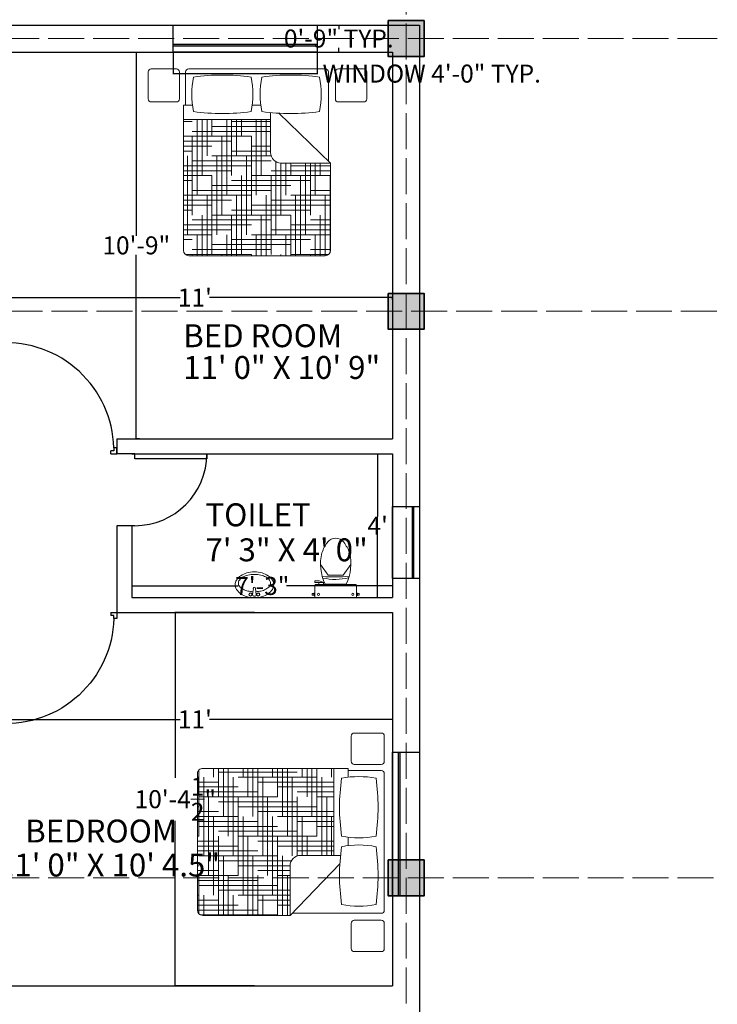
# Model space of a CAD drawing. Units: inches. Extents: x -113 to 5399, y -1393 to 3302.
# Tile 9 of 40: x 1194 to 1427, y 460 to 788. Entities that reach past the tile are written whole.
import ezdxf

# ---------------------------------------------------------------- set-up
doc = ezdxf.new("R2010")
doc.units = ezdxf.units.IN
doc.header["$MEASUREMENT"] = 0
doc.linetypes.add('ACAD_ISO02W100', pattern=[15, 12, -3])
for name, color, linetype, lineweight in [('A-ANNO-DIMS', 254, 'Continuous', 18), ('A-AREA-IDEN', 4, 'Continuous', 18), ('A-COLS', 7, 'Continuous', 35), ('A-FLOR-FIXT', 8, 'Continuous', 18), ('doors', 2, 'Continuous', 25), ('furniture', 131, 'Continuous', 18), ('GRIDS', 7, 'ACAD_ISO02W100', 13), ('walls', 1, 'Continuous', 25), ('windows', 3, 'Continuous', 25)]:
    doc.layers.add(name, color=color, linetype=linetype, lineweight=lineweight)
doc.styles.get("Standard").update_dxf_attribs({"font": 'arial.ttf'})
doc.dimstyles.get("Standard").update_dxf_attribs({"dimtxt": 6, "dimasz": 0.18, "dimexe": 0.18, "dimexo": 0.0625, "dimgap": 0.09, "dimtad": 0, "dimtih": 1, "dimtoh": 1, "dimdec": 1, "dimzin": 0, "dimdsep": 46, "dimlunit": 4, "dimtxsty": 'Standard', "dimblk": 'ARCHTICK', "dimcen": 0.09, "dimadec": 0, "dimazin": 0, "dimtfac": 1, "dimtdec": 1, "dimtofl": 0, "dimtmove": 0, "dimatfit": 3, "dimfxl": 1, "dimtolj": 1, "dimtzin": 0, "dimarcsym": 0})

# ---------------------------------------------------------------- blocks, each defined once
blk = doc.blocks.new('*U2')
for p, q in [((0, 0), (0, -6)), ((24, 0), (24, -6))]:
    blk.add_line(p, q)
blk.add_lwpolyline([(0, 0), (0, 24), (1.75, 24), (1.75, 0)], close=True)
blk.add_arc((0, 0), 24, 0, 90)
blk = doc.blocks.new('*X4')
at = {"color": 0}
for p, q in [((4.3594, 18.5625), (4.3594, 18.6457)), ((4.5, 18), (4.5, 18.6457)), ((4.5469, 18.1875), (4.5469, 18.6457)), ((4.5938, 18.375), (4.5938, 18.6457)), ((4.6406, 18.5625), (4.6406, 18.6457)), ((4.6875, 18.6094), (5.4375, 18.6094)), ((4.7812, 18), (4.7812, 18.6457)), ((4.8281, 18.1875), (4.8281, 18.6457)), ((4.875, 18.375), (4.875, 18.6457)), ((4.9219, 18.5625), (4.9219, 18.6457)), ((5.0625, 18), (5.0625, 18.6457)), ((5.1094, 18.1875), (5.1094, 18.6457)), ((5.1562, 18.375), (5.1562, 18.6457)), ((5.2031, 18.5625), (5.2031, 18.6457)), ((5.3438, 18), (5.3438, 18.6457)), ((5.3906, 18.1875), (5.3906, 18.6457)), ((5.4375, 18.375), (5.4375, 18.6457)), ((5.4844, 18.5625), (5.4844, 18.6457)), ((5.625, 18), (5.625, 18.6287)), ((4.3395, 18.5156), (5.0625, 18.5156)), ((4.4531, 17.8169), (4.4531, 18.5625)), ((4.5, 18.5625), (5.25, 18.5625)), ((4.7344, 17.8125), (4.7344, 18.5625)), ((5.0156, 17.8125), (5.0156, 18.5625)), ((5.2969, 17.8125), (5.2969, 18.5625)), ((5.4375, 18.5156), (5.6375, 18.5156)), ((5.5781, 17.8125), (5.5781, 18.5625)), ((5.625, 18.5625), (5.6375, 18.5625)), ((4.3395, 18.4688), (4.875, 18.4688)), ((4.3395, 18.4219), (4.6875, 18.4219)), ((5.0625, 18.4219), (5.6375, 18.4219)), ((5.25, 18.4688), (5.6375, 18.4688)), ((4.3395, 18.375), (4.5, 18.375)), ((4.4062, 17.8169), (4.4062, 18.375)), ((4.6875, 17.8114), (4.6875, 18.375)), ((4.6875, 18.3281), (5.4375, 18.3281)), ((4.875, 18.375), (5.625, 18.375)), ((4.9688, 17.625), (4.9688, 18.375)), ((5.25, 17.625), (5.25, 18.375)), ((5.5312, 17.625), (5.5312, 18.375)), ((4.3395, 18.2344), (5.0625, 18.2344)), ((4.5, 18.2812), (5.25, 18.2812)), ((5.4375, 18.2344), (5.6375, 18.2344)), ((5.625, 18.2812), (5.6375, 18.2812)), ((4.3395, 18.1875), (4.875, 18.1875)), ((4.3395, 18.1406), (4.6875, 18.1406)), ((4.3594, 17.8169), (4.3594, 18.1875)), ((4.6406, 17.8169), (4.6406, 18.1875)), ((4.9219, 17.4375), (4.9219, 18.1875)), ((5.0625, 18.1406), (5.6375, 18.1406)), ((5.2031, 17.4375), (5.2031, 18.1875)), ((5.25, 18.1875), (5.6375, 18.1875)), ((5.4844, 17.4375), (5.4844, 18.1875)), ((4.3395, 18.0938), (4.5, 18.0938)), ((4.6875, 18.0469), (5.4375, 18.0469)), ((4.875, 18.0938), (5.625, 18.0938)), ((4.3395, 17.9531), (5.0625, 17.9531)), ((4.5, 18), (5.25, 18)), ((4.5938, 17.8169), (4.5938, 18)), ((4.875, 17.25), (4.875, 18)), ((5.1562, 17.25), (5.1562, 18)), ((5.4375, 17.25), (5.4375, 18)), ((5.4375, 17.9531), (5.6375, 17.9531)), ((5.625, 18), (5.6375, 18)), ((4.3395, 17.9062), (4.875, 17.9062)), ((4.3395, 17.8594), (4.6875, 17.8594)), ((5.0625, 17.8594), (5.6375, 17.8594)), ((5.25, 17.9062), (5.6375, 17.9062)), ((4.7421, 17.7656), (5.4375, 17.7656)), ((4.8281, 17.2457), (4.8281, 17.8125)), ((4.875, 17.8125), (5.625, 17.8125)), ((5.1094, 17.2457), (5.1094, 17.8125)), ((5.3906, 17.2457), (5.3906, 17.8125)), ((4.7548, 17.7188), (5.25, 17.7188)), ((4.7548, 17.6719), (5.0625, 17.6719)), ((5.4375, 17.6719), (5.6375, 17.6719)), ((5.625, 17.7188), (5.6375, 17.7188)), ((4.7548, 17.625), (4.875, 17.625)), ((4.7812, 17.2457), (4.7812, 17.625)), ((5.0625, 17.2457), (5.0625, 17.625)), ((5.0625, 17.5781), (5.6375, 17.5781)), ((5.25, 17.625), (5.6375, 17.625)), ((5.3438, 17.2457), (5.3438, 17.625)), ((5.625, 17.2627), (5.625, 17.625)), ((4.7548, 17.4844), (5.4375, 17.4844)), ((4.875, 17.5312), (5.625, 17.5312)), ((4.7548, 17.4375), (5.25, 17.4375)), ((4.7548, 17.3906), (5.0625, 17.3906)), ((5.0156, 17.2457), (5.0156, 17.4375)), ((5.2969, 17.2457), (5.2969, 17.4375)), ((5.4375, 17.3906), (5.6375, 17.3906)), ((5.5781, 17.2457), (5.5781, 17.4375)), ((5.625, 17.4375), (5.6375, 17.4375)), ((4.7548, 17.3438), (4.875, 17.3438)), ((5.0625, 17.2969), (5.6375, 17.2969)), ((5.25, 17.3438), (5.6375, 17.3438)), ((4.875, 17.25), (5.6077, 17.25)), ((4.9688, 17.2457), (4.9688, 17.25)), ((5.25, 17.2457), (5.25, 17.25)), ((5.5312, 17.2457), (5.5312, 17.25))]:
    blk.add_line(p, q, dxfattribs=at)
blk = doc.blocks.new('MAT-P01')
for p, q in [((0.0087, 0.8464), (0.2471, 0.8464)), ((0.3737, 0.8464), (1.6737, 0.8464)), ((1.7922, 0.8464), (2.0306, 0.8464)), ((-0.0213, 0.8164), (-0.0213, 0.5605)), ((0.2771, 0.8164), (0.2771, 0.5605)), ((0.3437, 0.8164), (0.3437, -0.0316)), ((1.7037, 0.8164), (1.7037, 0.5005)), ((1.7622, 0.8164), (1.7622, 0.5605)), ((2.0606, 0.8164), (2.0606, 0.5605)), ((0.0087, 0.5305), (0.2471, 0.5305)), ((0.9879, 0.5005), (1.0693, 0.5005)), ((1.6393, 0.5005), (1.7237, 0.5005)), ((1.7237, 0.5005), (1.7237, -0.8836)), ((1.7922, 0.5305), (2.0306, 0.5305)), ((0.8146, 0.423), (0.3237, -0.0509)), ((0.8949, 0.4293), (0.8949, 0.0491)), ((0.8949, 0.3643), (1.7237, 0.3643)), ((0.8949, 0.3643), (0.8949, 0.0491)), ((0.8949, 0.3643), (1.7237, 0.3643)), ((1.7237, 0.3643), (1.7237, -0.8836)), ((0.3237, -0.0509), (0.7949, -0.0509)), ((0.3237, -0.0509), (0.3237, -0.8836)), ((0.3737, -0.9336), (1.6737, -0.9336))]:
    blk.add_line(p, q)
for centre, radius, start, end in [((0.0087, 0.8164), 0.03, 90, 180), ((0.2471, 0.8164), 0.03, 0, 90), ((0.3737, 0.8164), 0.03, 90, 180), ((1.6737, 0.8164), 0.03, 0, 90), ((1.7922, 0.8164), 0.03, 90, 180), ((2.0306, 0.8164), 0.03, 0, 90), ((1.2251, 0.6034), 0.8138, 168.37298, 191.62702), ((0.7029, -1.1436), 1.9306, 81.81622, 98.18378), ((0.1806, 0.6034), 0.8138, 348.37298, 11.62702), ((1.8766, 0.6034), 0.8138, 168.37298, 191.62702), ((1.3543, -1.1436), 1.9306, 81.81622, 98.18378), ((0.8321, 0.6034), 0.8138, 348.37298, 11.62702), ((0.0087, 0.5605), 0.03, 180, 270), ((0.2471, 0.5605), 0.03, 270, 0), ((1.7922, 0.5605), 0.03, 180, 270), ((2.0306, 0.5605), 0.03, 270, 0), ((0.7029, 2.3504), 1.9306, 261.81622, 278.18378), ((1.3543, 2.3504), 1.9306, 261.81622, 278.18378), ((0.7949, 0.0491), 0.1, 270, 0), ((0.3737, -0.8836), 0.05, 180, 270), ((1.6737, -0.8836), 0.05, 270, 0)]:
    blk.add_arc(centre, radius, start, end)
at = {"rotation": 270}
blk.add_blockref('*X4', (-16.9221, 4.7038), dxfattribs=at)
blk = doc.blocks.new('toilet-3')
at = {"color": 0, "linetype": 'ByBlock'}
for p, q in [((-0.281, -0.05), (-0.281, -0.069)), ((-0.281, -0.05), (-0.261, -0.05)), ((-0.281, -0.069), (-0.261, -0.069)), ((-0.261, -0.047), (-0.261, -0.072)), ((-0.261, -0.047), (-0.251, -0.047)), ((-0.261, -0.072), (-0.251, -0.072)), ((-0.251, -0.047), (-0.251, -0.072)), ((-0.25, -0.03), (-0.25, -0.165)), ((0.24, -0.02), (-0.24, -0.02)), ((0.25, -0.03), (0.25, -0.165)), ((0.261, -0.047), (0.251, -0.047)), ((0.251, -0.047), (0.251, -0.072)), ((0.261, -0.072), (0.251, -0.072)), ((0.261, -0.047), (0.261, -0.072)), ((0.281, -0.05), (0.261, -0.05)), ((0.281, -0.069), (0.261, -0.069)), ((0.281, -0.05), (0.281, -0.069)), ((-0.144, -0.2), (-0.25, -0.2)), ((-0.25, -0.2), (-0.25, -0.222)), ((-0.198, -0.222), (-0.25, -0.222)), ((0.24, -0.175), (-0.24, -0.175)), ((-0.202, -0.2), (-0.202, -0.175)), ((-0.198, -0.222), (-0.16, -0.207)), ((-0.16, -0.207), (-0.16, -0.2)), ((-0.144, -0.2), (-0.144, -0.175)), ((0.125, -0.182), (-0.125, -0.182)), ((-0.089, -0.287), (-0.18, -0.415)), ((0.089, -0.287), (-0.089, -0.287)), ((0.089, -0.287), (0.18, -0.415))]:
    blk.add_line(p, q, dxfattribs=at)
for centre in [(-0.205, -0.059), (0.205, -0.059)]:
    blk.add_circle(centre, 0.0125, dxfattribs=at)
for centre, radius, start, end in [((-0.24, -0.03), 0.01, 90, 180), ((0.24, -0.03), 0.01, 0, 90), ((-0.24, -0.165), 0.01, 180, 270), ((0.376, -0.424), 0.557, 154.2321, 193.6755), ((-0.376, -0.424), 0.557, 346.3245, 25.7679), ((0.24, -0.165), 0.01, 270, 0), ((-0.013, -1.787), 1.521, 83.4552, 95.5271), ((-0.005, -0.896), 0.659, 75.9276, 103.0204), ((0.262, -0.406), 0.452, 199.2942, 217.2549), ((-0.265, -0.4), 0.457, 322.2382, 340.1051), ((-0.001, -0.609), 0.12, 216.3794, 323.6206)]:
    blk.add_arc(centre, radius, start, end, dxfattribs=at)
blk = doc.blocks.new('wash-6')
at = {"color": 0, "linetype": 'ByBlock'}
for p, q in [((-0.036, -0.063), (-0.021, -0.18)), ((0.036, -0.063), (0.021, -0.18))]:
    blk.add_line(p, q, dxfattribs=at)
for centre, radius in [((-0.075, -0.062), 0.0325), ((-0.075, -0.062), 0.0263), ((0.075, -0.062), 0.0325), ((0.075, -0.062), 0.0263)]:
    blk.add_circle(centre, radius, dxfattribs=at)
for centre, radius, start, end in [((0, -0.56), 0.56, 90, 105.4371), ((-0.204, -0.25), 0.17, 148.1465, 180), ((-0.107, -0.311), 0.285, 123.6901, 148.1465), ((-0.114, -0.361), 0.225, 118.369, 142.5096), ((-0.042, -0.407), 0.401, 105.4371, 123.6901), ((-0.045, -0.488), 0.37, 102.6081, 118.369), ((0, -0.69), 0.576, 92.9466, 102.6081), ((0, -0.063), 0.0361, 0, 180), ((0, -0.18), 0.0215, 180, 0), ((0, -0.56), 0.56, 74.5629, 90), ((0, -0.69), 0.576, 77.3919, 87.0534), ((0.045, -0.488), 0.37, 61.631, 77.3919), ((0.042, -0.407), 0.401, 56.3099, 74.5629), ((0.114, -0.361), 0.225, 37.4904, 61.631), ((0.107, -0.311), 0.285, 31.8535, 56.3099), ((0.204, -0.25), 0.17, 0, 31.8535), ((-0.204, -0.25), 0.17, 180, 211.8535), ((-0.107, -0.189), 0.285, 211.8535, 236.3099), ((-0.217, -0.282), 0.0954, 142.5096, 180), ((-0.217, -0.282), 0.0954, 180, 217.4904), ((-0.114, -0.203), 0.225, 217.4904, 241.631), ((0.114, -0.203), 0.225, 298.369, 322.5096), ((0.107, -0.189), 0.285, 303.6901, 328.1465), ((0.217, -0.282), 0.0954, 0, 37.4904), ((0.217, -0.282), 0.0954, 322.5096, 0), ((0.204, -0.25), 0.17, 328.1465, 0), ((-0.042, -0.092), 0.401, 236.3099, 254.5629), ((-0.045, -0.076), 0.37, 241.631, 257.3919), ((0, 0.06), 0.56, 254.5629, 270), ((0, 0.125), 0.576, 257.3919, 270), ((0, 0.125), 0.576, 270, 282.6081), ((0, 0.06), 0.56, 270, 285.4371), ((0.045, -0.076), 0.37, 282.6081, 298.369), ((0.042, -0.092), 0.401, 285.4371, 303.6901)]:
    blk.add_arc(centre, radius, start, end, dxfattribs=at)
blk = doc.blocks.new('_ArchTick')
at = {"color": 0, "linetype": 'ByBlock', "const_width": 0.15}
blk.add_lwpolyline([(-0.5, -0.5), (0.5, 0.5)], dxfattribs=at)
blk = doc.blocks.new('*D39')
at = {"layer": 'A-ANNO-DIMS', "color": 0, "lineweight": -2, "transparency": 16777216}
for p, q in [((1223.9, 777.53), (1232.87, 777.53)), ((1232.69, 777.53), (1232.69, 716.19)), ((1232.69, 648.53), (1232.69, 709.88)), ((1233.79, 648.53), (1232.51, 648.53))]:
    blk.add_line(p, q, dxfattribs=at)
at = {"layer": 'Defpoints', "color": 0, "transparency": 16777216}
for p in [(1223.84, 777.53), (1232.69, 648.53), (1233.85, 648.53)]:
    blk.add_point(p, dxfattribs=at)
at = {"layer": 'A-ANNO-DIMS', "color": 0, "lineweight": -2, "transparency": 16777216, "xscale": 0.18, "yscale": 0.18, "zscale": 0.18}
for p, rotation in [((1232.69, 777.53), 90), ((1232.69, 648.53), 270)]:
    blk.add_blockref('_ArchTick', p, dxfattribs=dict(at, rotation=rotation))
at = {"layer": 'A-ANNO-DIMS', "color": 0, "transparency": 16777216, "insert": (1232.69, 713.03), "char_height": 6, "attachment_point": 5}
blk.add_mtext('\\A1;10\'-9"', dxfattribs=at)
blk = doc.blocks.new('*D40')
at = {"layer": 'A-ANNO-DIMS', "color": 0, "lineweight": -2, "transparency": 16777216}
for p, q in [((1186.23, 695), (1186.23, 695.81)), ((1186.23, 695.63), (1247.33, 695.63)), ((1318.23, 695.63), (1257.13, 695.63)), ((1318.23, 695), (1318.23, 695.81))]:
    blk.add_line(p, q, dxfattribs=at)
at = {"layer": 'Defpoints', "color": 0, "transparency": 16777216}
for p in [(1186.23, 695.63), (1186.23, 694.94), (1318.23, 694.94)]:
    blk.add_point(p, dxfattribs=at)
at = {"layer": 'A-ANNO-DIMS', "color": 0, "lineweight": -2, "transparency": 16777216, "xscale": 0.18, "yscale": 0.18, "zscale": 0.18, "rotation": 180}
blk.add_blockref('_ArchTick', (1186.23, 695.63), dxfattribs=at)
at = {"layer": 'A-ANNO-DIMS', "color": 0, "lineweight": -2, "transparency": 16777216, "xscale": 0.18, "yscale": 0.18, "zscale": 0.18}
blk.add_blockref('_ArchTick', (1318.23, 695.63), dxfattribs=at)
at = {"layer": 'A-ANNO-DIMS', "color": 0, "transparency": 16777216, "insert": (1252.23, 695.63), "char_height": 6, "attachment_point": 5}
blk.add_mtext("\\A1;11'", dxfattribs=at)
blk = doc.blocks.new('*D45')
at = {"layer": 'A-ANNO-DIMS', "color": 0, "lineweight": -2, "transparency": 16777216}
for p, q in [((1272.17, 590.53), (1245.54, 590.53)), ((1245.72, 590.53), (1245.72, 535.45)), ((1245.72, 466.03), (1245.72, 521.12)), ((1272.17, 466.03), (1245.54, 466.03))]:
    blk.add_line(p, q, dxfattribs=at)
at = {"layer": 'Defpoints', "color": 0, "transparency": 16777216}
for p in [(1272.23, 590.53), (1245.72, 466.03), (1272.23, 466.03)]:
    blk.add_point(p, dxfattribs=at)
at = {"layer": 'A-ANNO-DIMS', "color": 0, "lineweight": -2, "transparency": 16777216, "xscale": 0.18, "yscale": 0.18, "zscale": 0.18}
for p, rotation in [((1245.72, 590.53), 90), ((1245.72, 466.03), 270)]:
    blk.add_blockref('_ArchTick', p, dxfattribs=dict(at, rotation=rotation))
at = {"layer": 'A-ANNO-DIMS', "color": 0, "transparency": 16777216, "insert": (1245.72, 528.28), "char_height": 6, "attachment_point": 5}
blk.add_mtext('\\A1;10\'-4{\\H1x;\\S1/2;}"', dxfattribs=at)
blk = doc.blocks.new('*D46')
at = {"layer": 'A-ANNO-DIMS', "color": 0, "lineweight": -2, "transparency": 16777216}
for p, q in [((1186.23, 554.92), (1186.23, 554.73)), ((1186.23, 554.91), (1247.33, 554.91)), ((1318.23, 554.91), (1257.13, 554.91)), ((1318.23, 554.92), (1318.23, 554.73))]:
    blk.add_line(p, q, dxfattribs=at)
at = {"layer": 'Defpoints', "color": 0, "transparency": 16777216}
for p in [(1186.23, 554.98), (1186.23, 554.91), (1318.23, 554.98)]:
    blk.add_point(p, dxfattribs=at)
at = {"layer": 'A-ANNO-DIMS', "color": 0, "lineweight": -2, "transparency": 16777216, "xscale": 0.18, "yscale": 0.18, "zscale": 0.18, "rotation": 180}
blk.add_blockref('_ArchTick', (1186.23, 554.91), dxfattribs=at)
at = {"layer": 'A-ANNO-DIMS', "color": 0, "lineweight": -2, "transparency": 16777216, "xscale": 0.18, "yscale": 0.18, "zscale": 0.18}
blk.add_blockref('_ArchTick', (1318.23, 554.91), dxfattribs=at)
at = {"layer": 'A-ANNO-DIMS', "color": 0, "transparency": 16777216, "insert": (1252.23, 554.91), "char_height": 6, "attachment_point": 5}
blk.add_mtext("\\A1;11'", dxfattribs=at)
blk = doc.blocks.new('*D47')
at = {"layer": 'A-ANNO-DIMS', "color": 0, "lineweight": -2, "transparency": 16777216}
for p, q in [((1312.97, 643.53), (1313.39, 643.53)), ((1313.21, 643.53), (1313.21, 622.62)), ((1313.21, 595.53), (1313.21, 616.44)), ((1312.97, 595.53), (1313.39, 595.53))]:
    blk.add_line(p, q, dxfattribs=at)
at = {"layer": 'Defpoints', "color": 0, "transparency": 16777216}
for p in [(1312.91, 643.53), (1312.91, 595.53), (1313.21, 595.53)]:
    blk.add_point(p, dxfattribs=at)
at = {"layer": 'A-ANNO-DIMS', "color": 0, "lineweight": -2, "transparency": 16777216, "xscale": 0.18, "yscale": 0.18, "zscale": 0.18}
for p, rotation in [((1313.21, 643.53), 90), ((1313.21, 595.53), 270)]:
    blk.add_blockref('_ArchTick', p, dxfattribs=dict(at, rotation=rotation))
at = {"layer": 'A-ANNO-DIMS', "color": 0, "transparency": 16777216, "insert": (1313.21, 619.53), "char_height": 6, "attachment_point": 5}
blk.add_mtext("\\A1;4'", dxfattribs=at)
blk = doc.blocks.new('*D48')
at = {"layer": 'A-ANNO-DIMS', "color": 0, "lineweight": -2, "transparency": 16777216}
for p, q in [((1231.23, 599.86), (1231.23, 599.24)), ((1231.23, 599.42), (1266.69, 599.42)), ((1318.23, 599.42), (1282.77, 599.42)), ((1318.23, 599.86), (1318.23, 599.24))]:
    blk.add_line(p, q, dxfattribs=at)
at = {"layer": 'Defpoints', "color": 0, "transparency": 16777216}
for p in [(1231.23, 599.92), (1231.23, 599.42), (1318.23, 599.92)]:
    blk.add_point(p, dxfattribs=at)
at = {"layer": 'A-ANNO-DIMS', "color": 0, "lineweight": -2, "transparency": 16777216, "xscale": 0.18, "yscale": 0.18, "zscale": 0.18, "rotation": 180}
blk.add_blockref('_ArchTick', (1231.23, 599.42), dxfattribs=at)
at = {"layer": 'A-ANNO-DIMS', "color": 0, "lineweight": -2, "transparency": 16777216, "xscale": 0.18, "yscale": 0.18, "zscale": 0.18}
blk.add_blockref('_ArchTick', (1318.23, 599.42), dxfattribs=at)
at = {"layer": 'A-ANNO-DIMS', "color": 0, "transparency": 16777216, "insert": (1274.73, 599.42), "char_height": 6, "attachment_point": 5}
blk.add_mtext('\\A1;7\'-3"', dxfattribs=at)
blk = doc.blocks.new('WIN-PLAN-48IN')
h = blk.add_hatch(color=256)
h.dxf.hatch_style = 1
h.paths.add_polyline_path([(48, 2.5), (0, 2.5), (0, 2), (48, 2)])
for p, q in [((0, 9), (48, 9)), ((0, 0), (0, 9)), ((48, 9), (48, 0)), ((48, 2.5), (0, 2.5)), ((48, 2), (0, 2)), ((48, 0), (0, 0))]:
    blk.add_line(p, q)
blk = doc.blocks.new('WIN-PLAN-24IN')
h = blk.add_hatch(color=256)
h.dxf.hatch_style = 1
h.paths.add_polyline_path([(6.5, 24), (6.5, 0), (7, 0), (7, 24)])
for p, q in [((0, 0), (0, 24)), ((0, 24), (9, 24)), ((6.5, 24), (6.5, 0)), ((7, 24), (7, 0)), ((9, 24), (9, 0)), ((9, 0), (0, 0))]:
    blk.add_line(p, q)
blk = doc.blocks.new('COLUMN-12IN-SQUARE')
h = blk.add_hatch(color=256)
h.dxf.hatch_style = 1
h.paths.add_polyline_path([(6, 6), (-6, 6), (-6, -6), (6, -6)])
blk.add_lwpolyline([(-6, 6), (6, 6), (6, -6), (-6, -6)], close=True)
blk = doc.blocks.new('DOOR-SINGLE-36IN-PLAN')
for p, q in [((0.5, 2), (0.5, 36.98)), ((0.5, 36.98), (1.5, 36.98)), ((1.5, 36.98), (1.5, 2)), ((0, 2), (0, 0)), ((0, 2), (1.04, 2)), ((1.5, 2), (0.5, 2)), ((1.04, 2), (1.04, 0.98)), ((1.04, 0.98), (2, 0.98)), ((2, 0), (2, 0.98)), ((38.96, 0.98), (38, 0.98)), ((38, 0), (38, 0.98)), ((40, 2), (38.96, 2)), ((38.96, 2), (38.96, 0.98)), ((40, 0), (40, 2)), ((0, 0), (2, 0)), ((0, 0), (2, 0)), ((38, 0), (40, 0))]:
    blk.add_line(p, q)
blk.add_arc((2.94, 0.99), 36.04, 1.6003, 93.0893)
blk = doc.blocks.new('*D173')
at = {"layer": 'A-ANNO-DIMS', "color": 0, "lineweight": -2, "transparency": 16777216}
for p, q in [((1245.05, 777.47), (1245.05, 770.15)), ((1293.05, 777.47), (1293.05, 770.15)), ((1245.05, 770.33), (1293.05, 770.33)), ((1293.05, 770.33), (1293.23, 770.33))]:
    blk.add_line(p, q, dxfattribs=at)
at = {"layer": 'Defpoints', "color": 0, "transparency": 16777216}
for p in [(1245.05, 777.53), (1293.05, 777.53), (1293.05, 770.33)]:
    blk.add_point(p, dxfattribs=at)
at = {"layer": 'A-ANNO-DIMS', "color": 0, "lineweight": -2, "transparency": 16777216, "xscale": 0.18, "yscale": 0.18, "zscale": 0.18, "rotation": 180}
blk.add_blockref('_ArchTick', (1245.05, 770.33), dxfattribs=at)
at = {"layer": 'A-ANNO-DIMS', "color": 0, "lineweight": -2, "transparency": 16777216, "xscale": 0.18, "yscale": 0.18, "zscale": 0.18}
blk.add_blockref('_ArchTick', (1293.05, 770.33), dxfattribs=at)
at = {"layer": 'A-ANNO-DIMS', "color": 0, "transparency": 16777216, "insert": (1331.28, 770.33), "char_height": 6, "attachment_point": 5}
blk.add_mtext('\\A1;WINDOW 4\'-0" TYP.', dxfattribs=at)
blk = doc.blocks.new('*D174')
at = {"layer": 'A-ANNO-DIMS', "color": 0, "lineweight": -2, "transparency": 16777216}
for p, q in [((1293.11, 786.53), (1300.43, 786.53)), ((1300.25, 786.53), (1300.25, 785.19)), ((1300.25, 777.53), (1300.25, 778.88)), ((1293.11, 777.53), (1300.43, 777.53))]:
    blk.add_line(p, q, dxfattribs=at)
at = {"layer": 'Defpoints', "color": 0, "transparency": 16777216}
for p in [(1293.05, 786.53), (1300.25, 786.53), (1293.05, 777.53)]:
    blk.add_point(p, dxfattribs=at)
at = {"layer": 'A-ANNO-DIMS', "color": 0, "lineweight": -2, "transparency": 16777216, "xscale": 0.18, "yscale": 0.18, "zscale": 0.18}
for p, rotation in [((1300.25, 786.53), 90), ((1300.25, 777.53), 270)]:
    blk.add_blockref('_ArchTick', p, dxfattribs=dict(at, rotation=rotation))
at = {"layer": 'A-ANNO-DIMS', "color": 0, "transparency": 16777216, "insert": (1300.25, 782.03), "char_height": 6, "attachment_point": 5}
blk.add_mtext('\\A1;0\'-9" TYP.', dxfattribs=at)

msp = doc.modelspace()

# ---------------------------------------------------------------- linework, layer by layer
at = {"layer": 'GRIDS'}
for p, q in [((1322.73, 922.09), (1322.73, 54.5)), ((768.3, 782.03), (1417.18, 782.03)), ((1417.18, 782.03), (1426.54, 782.03)), ((769.42, 691.03), (1426.54, 691.03)), ((768.3, 502.03), (1426.54, 502.03))]:
    msp.add_line(p, q, dxfattribs=at)
at = {"layer": 'walls'}
for p, q in [((1186.23, 786.53), (1327.23, 786.53)), ((1327.23, 786.53), (1327.23, 136.53)), ((1186.23, 777.53), (1318.23, 777.53)), ((1318.23, 777.53), (1318.23, 648.53)), ((1226.23, 648.53), (1226.23, 643.53)), ((1226.23, 648.53), (1318.23, 648.53)), ((1231.23, 643.53), (1226.23, 643.53)), ((1231.23, 643.53), (1318.23, 643.53)), ((1318.23, 643.53), (1318.23, 595.53)), ((1226.23, 619.53), (1226.23, 590.53)), ((1231.23, 619.53), (1226.23, 619.53)), ((1231.23, 619.53), (1231.23, 595.53)), ((1231.23, 595.53), (1318.23, 595.53)), ((1226.23, 590.53), (1318.23, 590.53)), ((1318.23, 590.53), (1318.23, 466.03)), ((1169.23, 466.03), (1318.23, 466.03))]:
    msp.add_line(p, q, dxfattribs=at)

# ---------------------------------------------------------------- block references
at = {"layer": 'A-COLS'}
for p in [(1322.73, 782.03), (1322.73, 691.03), (1322.73, 502.03)]:
    msp.add_blockref('COLUMN-12IN-SQUARE', p, dxfattribs=at)
at = {"layer": 'A-FLOR-FIXT', "rotation": 180}
for name, p, xscale, yscale, zscale in [('toilet-3', (1299.23, 594.97), -27.95492935005888, 27.95492935005888, 27.95492935005888), ('wash-6', (1272.11, 595.53), -17.16666334294967, 17.16666334294967, 17.16666334294967)]:
    msp.add_blockref(name, p, dxfattribs=dict(at, xscale=xscale, yscale=yscale, zscale=zscale))
at = {"layer": 'doors'}
msp.add_blockref('DOOR-SINGLE-36IN-PLAN', (1186.23, 643.53), dxfattribs=at)
at = {"layer": 'doors', "rotation": 270}
msp.add_blockref('*U2', (1232.23, 643.53), dxfattribs=at)
at = {"layer": 'doors', "extrusion": (0, 0, -1), "zscale": -1, "rotation": 180}
msp.add_blockref('DOOR-SINGLE-36IN-PLAN', (-1186.23, 590.53), dxfattribs=at)
at = {"layer": 'furniture', "xscale": -35.02364872074636, "yscale": 35.02364872074636, "zscale": 35.02364872074636}
msp.add_blockref('MAT-P01', (1308.83, 742.29), dxfattribs=at)
at = {"layer": 'furniture', "xscale": -35.02364872074636, "yscale": 35.02364872074636, "zscale": 35.02364872074636, "rotation": 270}
msp.add_blockref('MAT-P01', (1285.8, 478.19), dxfattribs=at)
at = {"layer": 'windows'}
for name, p in [('WIN-PLAN-48IN', (1245.05, 777.53)), ('WIN-PLAN-24IN', (1318.23, 601.91))]:
    msp.add_blockref(name, p, dxfattribs=at)
at = {"layer": 'windows', "rotation": 269.999999999999}
msp.add_blockref('WIN-PLAN-48IN', (1318.23, 543.95), dxfattribs=at)

# ---------------------------------------------------------------- texts
at = {"layer": 'A-AREA-IDEN'}
for s, height, p in [('BED ROOM', 7.647, (1248.34, 679.07)), ('11\' 0" X 10\' 9"', 7.6473, (1248.34, 668.48)), ('TOILET', 7.647, (1255.77, 619.32)), ('7\' 3" X 4\' 0"', 7.6473, (1255.77, 607.64)), ('BEDROOM', 7.647, (1195.62, 513.84)), ('11\' 0" X 10\' 4.5"', 7.6473, (1186.23, 502.5))]:
    msp.add_text(s, height=height, dxfattribs=at).set_placement(p)

# ---------------------------------------------------------------- dimensions: what is measured, and where the dimension line sits
at = {"layer": 'A-ANNO-DIMS'}
dim = msp.add_linear_dim(base=(1300.25, 786.53), p1=(1293.05, 777.53), p2=(1293.05, 786.53), angle=90, text='<> TYP.', dimstyle='Standard', override={"dimdec": 1, "dimlfac": 1, "dimrnd": 0, "dimzin": 1, "dimdsep": 46, "dimlunit": 4, "dimfrac": 2}, dxfattribs=at)
dim.commit()
dim.dimension.update_dxf_attribs({"geometry": '*D174', "text_midpoint": (1300.25, 782.03)})
dim = msp.add_linear_dim(base=(1293.05, 770.33), p1=(1245.05, 777.53), p2=(1293.05, 777.53), text='WINDOW <> TYP.', dimstyle='Standard', override={"dimdec": 1, "dimlfac": 1, "dimrnd": 0, "dimzin": 1, "dimdsep": 46, "dimlunit": 4, "dimfrac": 2}, dxfattribs=at)
dim.commit()
dim.dimension.update_dxf_attribs({"geometry": '*D173', "text_midpoint": (1331.28, 770.33)})
for base, p1, p2, picture, middle in [((1232.69, 648.53), (1223.84, 777.53), (1233.85, 648.53), '*D39', (1232.69, 713.03)), ((1313.21, 595.53), (1312.91, 643.53), (1312.91, 595.53), '*D47', (1313.21, 619.53)), ((1245.72, 466.03), (1272.23, 590.53), (1272.23, 466.03), '*D45', (1245.72, 528.28))]:
    dim = msp.add_linear_dim(base=base, p1=p1, p2=p2, angle=90, dimstyle='Standard', override={"dimclrd": 0, "dimclre": 0, "dimclrt": 0}, dxfattribs=at)
    dim.commit()
    dim.dimension.update_dxf_attribs({"geometry": picture, "text_midpoint": middle})
for base, p1, p2, picture, middle in [((1186.23, 695.63), (1318.23, 694.94), (1186.23, 694.94), '*D40', (1252.23, 695.63)), ((1231.23, 599.42), (1318.23, 599.92), (1231.23, 599.92), '*D48', (1274.73, 599.42)), ((1186.23, 554.91), (1318.23, 554.98), (1186.23, 554.98), '*D46', (1252.23, 554.91))]:
    dim = msp.add_linear_dim(base=base, p1=p1, p2=p2, dimstyle='Standard', override={"dimclrd": 0, "dimclre": 0, "dimclrt": 0}, dxfattribs=at)
    dim.commit()
    dim.dimension.update_dxf_attribs({"geometry": picture, "text_midpoint": middle})

doc.saveas('drawing.dxf')
